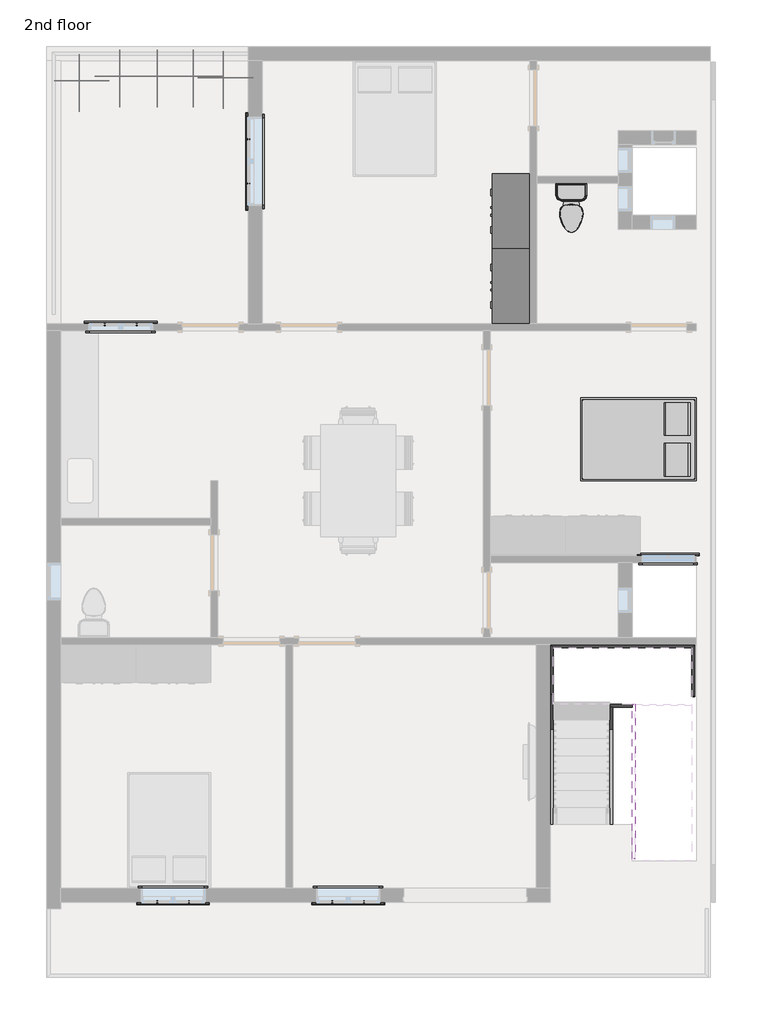
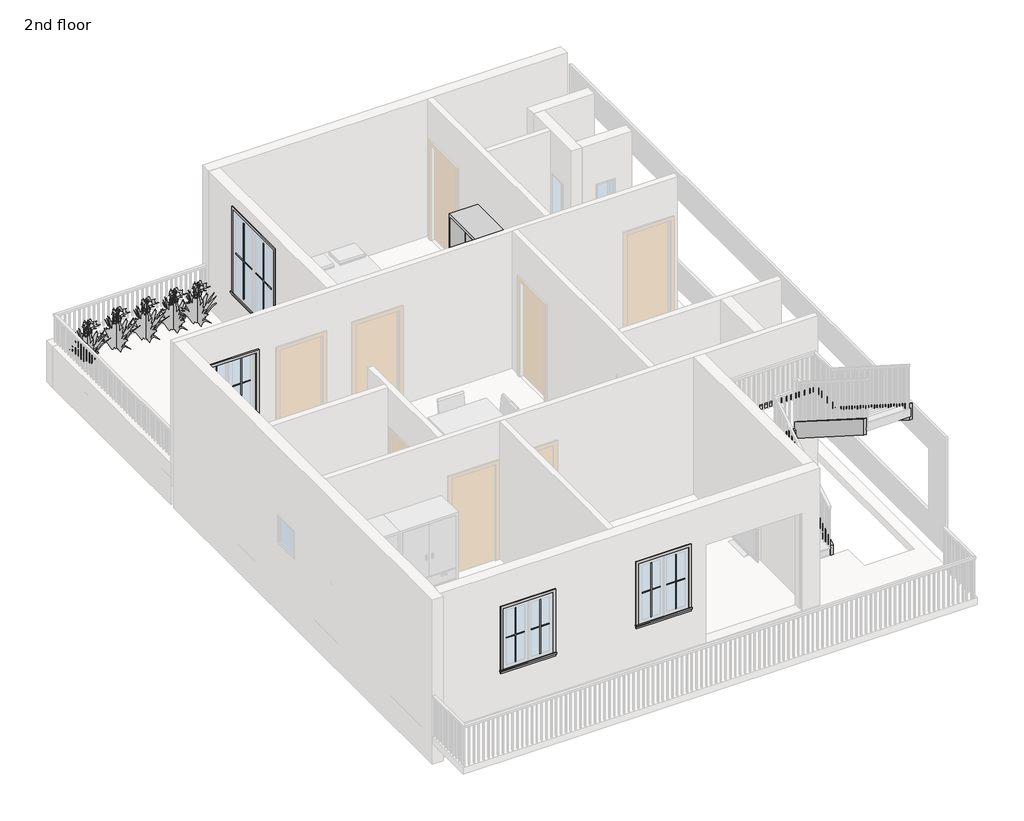
# One storey, part 5 of 5: 20 proxies, 8 members, 5 geographic elements, 3 furniture elements, 1 flow terminal.
"""IFC4 building model written with IfcOpenShell, lengths in millimetres."""

from ifc_helpers import new_model, si_unit, frame, origin, place, context, project, spatial, polyline, outline, extrude, faceted_brep, transform, mapped, element, save
from components import muntin_pattern_2x2_muntin_pattern_2x2_bff912c5, muntin_pattern_2x2_muntin_pattern_2x2_c2194282, muntin_pattern_2x2_muntin_pattern_2x2_88bf7f41, muntin_pattern_2x2_muntin_pattern_2x2_3dfd0a47, muntin_pattern_2x2_muntin_pattern_2x2_b3fe6957, muntin_pattern_2x2_muntin_pattern_2x2_3e0ecaf2, trim_window_exterior_flat_with_sill_e04b3088, trim_window_exterior_flat_with_sill_4930676f, trim_window_exterior_flat_with_sill_41619996, trim_window_interior_flat_picture_frame_2a7685fe, trim_window_interior_flat_picture_frame_dd064338, trim_window_interior_flat_picture_frame_51c85655, toilet_domestic_3d_toilet_domestic_3d_ba6479b0, toilet_domestic_3d_toilet_domestic_3d_30431060, furniture_b58f7881, furniture_82e269c4, rpc_plant_tropical_55f6ff97

model = new_model("IFC4")

# Units and contexts
model_context = context("Model", 3, world=origin())
ifc_project = project(units=[si_unit("LENGTHUNIT", "METRE", prefix="MILLI")], contexts=[model_context])

# Site, building, storey
site = spatial("IfcSite", under=ifc_project)
building = spatial("IfcBuilding", under=site)
storey = spatial("IfcBuildingStorey", under=building, Name="2nd floor", Elevation=7010.4)

# Proxies
placement = place(None, origin())
muntin_pattern_2x2_muntin_pattern_2x2_shape = muntin_pattern_2x2_muntin_pattern_2x2_bff912c5(model_context)
element("IfcBuildingElementProxy", 1, Name="Muntin Pattern_2x2 : Muntin Pattern_2x2", ObjectType="Muntin Pattern_2x2 : Muntin Pattern_2x2", at=placement, inside=storey, context=model_context, shape_type="MappedRepresentation", body=[
    mapped(muntin_pattern_2x2_muntin_pattern_2x2_shape, transform((-4824.2248597, 10579.5632925, 7994.65), x_axis=(0.0, 1.0, 0.0), y_axis=(-1.0, 0.0, 0.0), z_axis=(0.0, 0.0, 1.0))),
])
muntin_pattern_2x2_muntin_pattern_2x2_2_shape = muntin_pattern_2x2_muntin_pattern_2x2_c2194282(model_context)
element("IfcBuildingElementProxy", 2, Name="Muntin Pattern_2x2 : Muntin Pattern_2x2", ObjectType="Muntin Pattern_2x2 : Muntin Pattern_2x2", at=placement, inside=storey, context=model_context, shape_type="MappedRepresentation", body=[
    mapped(muntin_pattern_2x2_muntin_pattern_2x2_2_shape, transform((-4824.2248597, 11300.2882925, 7994.65), x_axis=(0.0, -1.0, 0.0), y_axis=(1.0, 0.0, 0.0), z_axis=(0.0, 0.0, 1.0))),
])
muntin_pattern_2x2_muntin_pattern_2x2_3_shape = muntin_pattern_2x2_muntin_pattern_2x2_88bf7f41(model_context)
element("IfcBuildingElementProxy", 3, Name="Muntin Pattern_2x2 : Muntin Pattern_2x2", ObjectType="Muntin Pattern_2x2 : Muntin Pattern_2x2", at=placement, inside=storey, context=model_context, shape_type="MappedRepresentation", body=[
    mapped(muntin_pattern_2x2_muntin_pattern_2x2_3_shape, transform((-7162.6123597, 8288.8007925, 7994.65), x_axis=(1.0, 0.0, 0.0), y_axis=(0.0, 1.0, 0.0), z_axis=(0.0, 0.0, 1.0))),
])
element("IfcBuildingElementProxy", 4, Name="Muntin Pattern_2x2 : Muntin Pattern_2x2", ObjectType="Muntin Pattern_2x2 : Muntin Pattern_2x2", at=placement, inside=storey, context=model_context, shape_type="MappedRepresentation", body=[
    mapped(muntin_pattern_2x2_muntin_pattern_2x2_3_shape, transform((-5794.1873597, -1102.8492075, 7994.65), x_axis=(-1.0, 0.0, 0.0), y_axis=(0.0, -1.0, 0.0), z_axis=(0.0, 0.0, 1.0))),
])
element("IfcBuildingElementProxy", 5, Name="Muntin Pattern_2x2 : Muntin Pattern_2x2", ObjectType="Muntin Pattern_2x2 : Muntin Pattern_2x2", at=placement, inside=storey, context=model_context, shape_type="MappedRepresentation", body=[
    mapped(muntin_pattern_2x2_muntin_pattern_2x2_3_shape, transform((-2946.0873597, -1102.8492075, 7994.65), x_axis=(-1.0, 0.0, 0.0), y_axis=(0.0, -1.0, 0.0), z_axis=(0.0, 0.0, 1.0))),
])
muntin_pattern_2x2_muntin_pattern_2x2_4_shape = muntin_pattern_2x2_muntin_pattern_2x2_3dfd0a47(model_context)
element("IfcBuildingElementProxy", 6, Name="Muntin Pattern_2x2 : Muntin Pattern_2x2", ObjectType="Muntin Pattern_2x2 : Muntin Pattern_2x2", at=placement, inside=storey, context=model_context, shape_type="MappedRepresentation", body=[
    mapped(muntin_pattern_2x2_muntin_pattern_2x2_4_shape, transform((-6645.0873597, 8288.8007925, 7994.65), x_axis=(-1.0, 0.0, 0.0), y_axis=(0.0, -1.0, 0.0), z_axis=(0.0, 0.0, 1.0))),
])
element("IfcBuildingElementProxy", 7, Name="Muntin Pattern_2x2 : Muntin Pattern_2x2", ObjectType="Muntin Pattern_2x2 : Muntin Pattern_2x2", at=placement, inside=storey, context=model_context, shape_type="MappedRepresentation", body=[
    mapped(muntin_pattern_2x2_muntin_pattern_2x2_4_shape, transform((-6311.7123597, -1102.8492075, 7994.65), x_axis=(1.0, 0.0, 0.0), y_axis=(0.0, 1.0, 0.0), z_axis=(0.0, 0.0, 1.0))),
])
element("IfcBuildingElementProxy", 8, Name="Muntin Pattern_2x2 : Muntin Pattern_2x2", ObjectType="Muntin Pattern_2x2 : Muntin Pattern_2x2", at=placement, inside=storey, context=model_context, shape_type="MappedRepresentation", body=[
    mapped(muntin_pattern_2x2_muntin_pattern_2x2_4_shape, transform((-3463.6123597, -1102.8492075, 7994.65), x_axis=(1.0, 0.0, 0.0), y_axis=(0.0, 1.0, 0.0), z_axis=(0.0, 0.0, 1.0))),
])
muntin_pattern_2x2_muntin_pattern_2x2_5_shape = muntin_pattern_2x2_muntin_pattern_2x2_b3fe6957(model_context)
element("IfcBuildingElementProxy", 9, Name="Muntin Pattern_2x2 : Muntin Pattern_2x2", ObjectType="Muntin Pattern_2x2 : Muntin Pattern_2x2", at=placement, inside=storey, context=model_context, shape_type="MappedRepresentation", body=[
    mapped(muntin_pattern_2x2_muntin_pattern_2x2_5_shape, transform((1784.5376403, 4516.9007925, 7385.05), x_axis=(1.0, 0.0, 0.0), y_axis=(0.0, 1.0, 0.0), z_axis=(0.0, 0.0, 1.0))),
])
muntin_pattern_2x2_muntin_pattern_2x2_6_shape = muntin_pattern_2x2_muntin_pattern_2x2_3e0ecaf2(model_context)
element("IfcBuildingElementProxy", 10, Name="Muntin Pattern_2x2 : Muntin Pattern_2x2", ObjectType="Muntin Pattern_2x2 : Muntin Pattern_2x2", at=placement, inside=storey, context=model_context, shape_type="MappedRepresentation", body=[
    mapped(muntin_pattern_2x2_muntin_pattern_2x2_6_shape, transform((2213.1626403, 4516.9007925, 7385.05), x_axis=(-1.0, 0.0, 0.0), y_axis=(0.0, -1.0, 0.0), z_axis=(0.0, 0.0, 1.0))),
])
trim_window_exterior_flat_with_sill_shape = trim_window_exterior_flat_with_sill_e04b3088(model_context)
element("IfcBuildingElementProxy", 11, Name="Trim-Window-Exterior-Flat : with Sill", ObjectType="Trim-Window-Exterior-Flat : with Sill", at=placement, inside=storey, context=model_context, shape_type="MappedRepresentation", body=[
    mapped(trim_window_exterior_flat_with_sill_shape, transform((-4833.7498597, 10939.9257925, 9753.6), x_axis=(0.0, -1.0, 0.0), y_axis=(0.0, 0.0, 1.0), z_axis=(-1.0, 0.0, 0.0))),
])
trim_window_exterior_flat_with_sill_2_shape = trim_window_exterior_flat_with_sill_4930676f(model_context)
element("IfcBuildingElementProxy", 12, Name="Trim-Window-Exterior-Flat : with Sill", ObjectType="Trim-Window-Exterior-Flat : with Sill", at=placement, inside=storey, context=model_context, shape_type="MappedRepresentation", body=[
    mapped(trim_window_exterior_flat_with_sill_2_shape, transform((-6903.8498597, 8298.3257925, 9271.0), x_axis=(-1.0, 0.0, 0.0), y_axis=(0.0, 0.0, 1.0), z_axis=(0.0, 1.0, 0.0))),
])
element("IfcBuildingElementProxy", 13, Name="Trim-Window-Exterior-Flat : with Sill", ObjectType="Trim-Window-Exterior-Flat : with Sill", at=placement, inside=storey, context=model_context, shape_type="MappedRepresentation", body=[
    mapped(trim_window_exterior_flat_with_sill_2_shape, transform((-6052.9498597, -1112.3742075, 9271.0), x_axis=(1.0, 0.0, 0.0), y_axis=(0.0, 0.0, 1.0), z_axis=(0.0, -1.0, 0.0))),
])
element("IfcBuildingElementProxy", 14, Name="Trim-Window-Exterior-Flat : with Sill", ObjectType="Trim-Window-Exterior-Flat : with Sill", at=placement, inside=storey, context=model_context, shape_type="MappedRepresentation", body=[
    mapped(trim_window_exterior_flat_with_sill_2_shape, transform((-3204.8498597, -1112.3742075, 9271.0), x_axis=(1.0, 0.0, 0.0), y_axis=(0.0, 0.0, 1.0), z_axis=(0.0, -1.0, 0.0))),
])
trim_window_exterior_flat_with_sill_3_shape = trim_window_exterior_flat_with_sill_41619996(model_context)
element("IfcBuildingElementProxy", 15, Name="Trim-Window-Exterior-Flat : with Sill", ObjectType="Trim-Window-Exterior-Flat : with Sill", at=placement, inside=storey, context=model_context, shape_type="MappedRepresentation", body=[
    mapped(trim_window_exterior_flat_with_sill_3_shape, transform((1998.8501403, 4526.4257925, 8229.6), x_axis=(-1.0, 0.0, 0.0), y_axis=(0.0, 0.0, 1.0), z_axis=(0.0, 1.0, 0.0))),
])
trim_window_interior_flat_picture_frame_shape = trim_window_interior_flat_picture_frame_2a7685fe(model_context)
element("IfcBuildingElementProxy", 16, Name="Trim-Window-Interior-Flat : Picture Frame", ObjectType="Trim-Window-Interior-Flat : Picture Frame", at=placement, inside=storey, context=model_context, shape_type="MappedRepresentation", body=[
    mapped(trim_window_interior_flat_picture_frame_shape, transform((-4605.1498597, 10939.9257925, 9753.6), x_axis=(0.0, 1.0, 0.0), y_axis=(0.0, 0.0, 1.0), z_axis=(1.0, 0.0, 0.0))),
])
trim_window_interior_flat_picture_frame_2_shape = trim_window_interior_flat_picture_frame_dd064338(model_context)
element("IfcBuildingElementProxy", 17, Name="Trim-Window-Interior-Flat : Picture Frame", ObjectType="Trim-Window-Interior-Flat : Picture Frame", at=placement, inside=storey, context=model_context, shape_type="MappedRepresentation", body=[
    mapped(trim_window_interior_flat_picture_frame_2_shape, transform((-6903.8498597, 8184.0257925, 9271.0), x_axis=(1.0, 0.0, 0.0), y_axis=(0.0, 0.0, 1.0), z_axis=(0.0, -1.0, 0.0))),
])
element("IfcBuildingElementProxy", 18, Name="Trim-Window-Interior-Flat : Picture Frame", ObjectType="Trim-Window-Interior-Flat : Picture Frame", at=placement, inside=storey, context=model_context, shape_type="MappedRepresentation", body=[
    mapped(trim_window_interior_flat_picture_frame_2_shape, transform((-6052.9498597, -883.7742075, 9271.0), x_axis=(-1.0, 0.0, 0.0), y_axis=(0.0, 0.0, 1.0), z_axis=(0.0, 1.0, 0.0))),
])
element("IfcBuildingElementProxy", 19, Name="Trim-Window-Interior-Flat : Picture Frame", ObjectType="Trim-Window-Interior-Flat : Picture Frame", at=placement, inside=storey, context=model_context, shape_type="MappedRepresentation", body=[
    mapped(trim_window_interior_flat_picture_frame_2_shape, transform((-3204.8498597, -883.7742075, 9271.0), x_axis=(-1.0, 0.0, 0.0), y_axis=(0.0, 0.0, 1.0), z_axis=(0.0, 1.0, 0.0))),
])
trim_window_interior_flat_picture_frame_3_shape = trim_window_interior_flat_picture_frame_51c85655(model_context)
element("IfcBuildingElementProxy", 20, Name="Trim-Window-Interior-Flat : Picture Frame", ObjectType="Trim-Window-Interior-Flat : Picture Frame", at=placement, inside=storey, context=model_context, shape_type="MappedRepresentation", body=[
    mapped(trim_window_interior_flat_picture_frame_3_shape, transform((1998.8501403, 4412.1257925, 8229.6), x_axis=(1.0, 0.0, 0.0), y_axis=(0.0, 0.0, 1.0), z_axis=(0.0, -1.0, 0.0))),
])

# Flow terminal
toilet_domestic_3d_toilet_domestic_3d_shape = toilet_domestic_3d_toilet_domestic_3d_ba6479b0(model_context)
toilet_domestic_3d_toilet_domestic_3d_2_shape = toilet_domestic_3d_toilet_domestic_3d_30431060(model_context)
element("IfcFlowTerminal", 21, ObjectType="Toilet-Domestic-3D : Toilet-Domestic-3D", at=placement, inside=storey, context=model_context, shape_type="MappedRepresentation", body=[
    mapped(toilet_domestic_3d_toilet_domestic_3d_shape, transform((424.0501403, 10089.0257925, 7010.4), x_axis=(1.0, 0.0, 0.0), y_axis=(0.0, 1.0, 0.0), z_axis=(0.0, 0.0, 1.0))),
    mapped(toilet_domestic_3d_toilet_domestic_3d_2_shape, transform((424.0501403, 10089.0257925, 7010.4), x_axis=(1.0, 0.0, 0.0), y_axis=(0.0, 1.0, 0.0), z_axis=(0.0, 0.0, 1.0))),
])

# Furniture
furniture_shape = furniture_b58f7881(model_context)
element("IfcFurniture", 22, ObjectType="Bed-Box : Double 53\" x 74\"", at=placement, inside=storey, context=model_context, shape_type="MappedRepresentation", body=[
    mapped(furniture_shape, transform((1750.6796485, 6757.8782516, 7010.4), x_axis=(0.0, -1.0, 0.0), y_axis=(1.0, 0.0, 0.0), z_axis=(0.0, 0.0, 1.0))),
])
furniture_2_shape = furniture_82e269c4(model_context)
element("IfcFurniture", 23, ObjectType="Wardrobe : 48\" x 72\" x 24\"", at=placement, inside=storey, context=model_context, shape_type="MappedRepresentation", body=[
    mapped(furniture_2_shape, transform((29.8889499, 8638.7325327, 7010.4), x_axis=(0.0, -1.0, 0.0), y_axis=(1.0, 0.0, 0.0), z_axis=(0.0, 0.0, 1.0))),
])
element("IfcFurniture", 24, ObjectType="Wardrobe : 48\" x 72\" x 24\"", at=placement, inside=storey, context=model_context, shape_type="MappedRepresentation", body=[
    mapped(furniture_2_shape, transform((29.8889499, 9857.9325327, 7010.4), x_axis=(0.0, -1.0, 0.0), y_axis=(1.0, 0.0, 0.0), z_axis=(0.0, 0.0, 1.0))),
])

# Geographic elements
rpc_plant_tropical_shape = rpc_plant_tropical_55f6ff97(model_context)
element("IfcGeographicElement", 25, ObjectType="RPC Plant - Tropical", at=placement, inside=storey, context=model_context, shape_type="MappedRepresentation", body=[
    mapped(rpc_plant_tropical_shape, transform((-7576.9498597, 12248.0257925, 7010.4), x_axis=(1.0, 0.0, 0.0), y_axis=(0.0, 1.0, 0.0), z_axis=(0.0, 0.0, 1.0))),
])
element("IfcGeographicElement", 26, ObjectType="RPC Plant - Tropical", at=placement, inside=storey, context=model_context, shape_type="MappedRepresentation", body=[
    mapped(rpc_plant_tropical_shape, transform((-5240.1498597, 12298.8257925, 7010.4), x_axis=(1.0, 0.0, 0.0), y_axis=(0.0, 1.0, 0.0), z_axis=(0.0, 0.0, 1.0))),
])
element("IfcGeographicElement", 27, ObjectType="RPC Plant - Tropical", at=placement, inside=storey, context=model_context, shape_type="MappedRepresentation", body=[
    mapped(rpc_plant_tropical_shape, transform((-6916.5498597, 12324.2257925, 7010.4), x_axis=(1.0, 0.0, 0.0), y_axis=(0.0, 1.0, 0.0), z_axis=(0.0, 0.0, 1.0))),
])
element("IfcGeographicElement", 28, ObjectType="RPC Plant - Tropical", at=placement, inside=storey, context=model_context, shape_type="MappedRepresentation", body=[
    mapped(rpc_plant_tropical_shape, transform((-6306.9498597, 12324.2257925, 7010.4), x_axis=(1.0, 0.0, 0.0), y_axis=(0.0, 1.0, 0.0), z_axis=(0.0, 0.0, 1.0))),
])
element("IfcGeographicElement", 29, ObjectType="RPC Plant - Tropical", at=placement, inside=storey, context=model_context, shape_type="MappedRepresentation", body=[
    mapped(rpc_plant_tropical_shape, transform((-5722.7498597, 12324.2257925, 7010.4), x_axis=(1.0, 0.0, 0.0), y_axis=(0.0, 1.0, 0.0), z_axis=(0.0, 0.0, 1.0))),
])

# Members
element("IfcMember", 30, ObjectType="Stringer - 2\" Width", at=placement, inside=storey, context=model_context, shape_type="SweptSolid", body=[
    extrude(outline(polyline([(157.6257925, 7010.4), (157.6257925, 7225.4106437), (2174.694781, 8509.0), (2263.4527505, 8204.2), (387.4813219, 7010.4), (157.6257925, 7010.4)])), frame((81.1501403, 0.0, 0.0), z_axis=(1.0, 0.0, 0.0), x_axis=(0.0, 1.0, 0.0)), (0.0, 0.0, 1.0), 50.8),
])
element("IfcMember", 31, ObjectType="Stringer - 2\" Width", at=placement, inside=storey, context=model_context, shape_type="SweptSolid", body=[
    extrude(outline(polyline([(157.6257925, 7010.4), (157.6257925, 7225.4106437), (2062.6257925, 8437.683371), (2062.6257925, 8076.4010268), (387.4813219, 7010.4), (157.6257925, 7010.4)])), frame((1046.3501403, 0.0, 0.0), z_axis=(1.0, 0.0, 0.0), x_axis=(0.0, 1.0, 0.0)), (0.0, 0.0, 1.0), 50.8),
])
element("IfcMember", 32, ObjectType="Stringer - 2\" Width", at=placement, inside=storey, context=model_context, shape_type="SweptSolid", body=[
    extrude(outline(polyline([(2331.5568041, 8509.0), (2242.7988346, 8204.2), (-401.1742075, 9886.7282995), (-401.1742075, 10248.0106437), (2331.5568041, 8509.0)])), frame((2379.8501403, 0.0, 0.0), z_axis=(1.0, 0.0, 0.0), x_axis=(0.0, 1.0, 0.0)), (0.0, 0.0, 1.0), 50.8),
])
element("IfcMember", 33, ObjectType="Stringer - 2\" Width", at=placement, inside=storey, context=model_context, shape_type="SweptSolid", body=[
    extrude(outline(polyline([(2113.4257925, 8647.8106437), (2113.4257925, 8286.5282995), (-401.1742075, 9886.7282995), (-401.1742075, 10248.0106437), (2113.4257925, 8647.8106437)])), frame((1414.6501403, 0.0, 0.0), z_axis=(1.0, 0.0, 0.0), x_axis=(0.0, 1.0, 0.0)), (0.0, 0.0, 1.0), 50.8),
])
element("IfcMember", 34, ObjectType="Stringer - 2\" Width", at=placement, inside=storey, context=model_context, shape_type="Brep", body=[
    faceted_brep([(2379.8501403, 2331.5568041, 8509.0), (2430.6501403, 2331.5568041, 8509.0), (2430.6501403, 3078.6257925, 8509.0), (2379.8501403, 3027.8257925, 8509.0), (2379.8501403, 2242.7988346, 8204.2), (2379.8501403, 3027.8257925, 8204.2), (2430.6501403, 2242.7988346, 8204.2), (2430.6501403, 3078.6257925, 8204.2)], [[[0, 1, 2, 3]], [[4, 0, 3, 5]], [[6, 4, 5, 7]], [[1, 6, 7, 2]], [[1, 0, 4, 6]], [[2, 7, 5, 3]]]),
])
element("IfcMember", 35, ObjectType="Stringer - 2\" Width", at=placement, inside=storey, context=model_context, shape_type="SweptSolid", body=[
    extrude(outline(polyline([(2430.6501403, 3078.6257925), (2379.8501403, 3027.8257925), (131.9501403, 3027.8257925), (81.1501403, 3078.6257925), (2430.6501403, 3078.6257925)])), frame((0.0, 0.0, 8204.2), z_axis=(0.0, 0.0, 1.0), x_axis=(1.0, 0.0, 0.0)), (0.0, 0.0, 1.0), 304.8),
])
element("IfcMember", 36, ObjectType="Stringer - 2\" Width", at=placement, inside=storey, context=model_context, shape_type="Brep", body=[
    faceted_brep([(131.9501403, 3027.8257925, 8509.0), (81.1501403, 3078.6257925, 8509.0), (81.1501403, 2174.694781, 8509.0), (131.9501403, 2174.694781, 8509.0), (131.9501403, 3027.8257925, 8204.2), (131.9501403, 2263.4527505, 8204.2), (81.1501403, 3078.6257925, 8204.2), (81.1501403, 2263.4527505, 8204.2)], [[[0, 1, 2, 3]], [[4, 0, 3, 5]], [[6, 4, 5, 7]], [[1, 6, 7, 2]], [[1, 0, 4, 6]], [[2, 7, 5, 3]]]),
])
element("IfcMember", 37, ObjectType="Stringer - 2\" Width", at=placement, inside=storey, context=model_context, shape_type="SweptSolid", body=[
    extrude(outline(polyline([(1046.3501403, 2062.6257925), (1046.3501403, 2113.4257925), (1414.6501403, 2113.4257925), (1414.6501403, 2062.6257925), (1046.3501403, 2062.6257925)])), frame((0.0, 0.0, 8204.2), z_axis=(0.0, 0.0, 1.0), x_axis=(1.0, 0.0, 0.0)), (0.0, 0.0, 1.0), 304.8),
])

save(model, "model.ifc")

# Revit data of these elements
# Type "Muntin Pattern_2x2 : Muntin Pattern_2x2"
#   Width [instance default] = 4' - 0"
#   Thickness = 0' - 0 1/2"
#   Height [instance default] = 4' - 0"
#   Distance = 0' - 0 3/4"
#   Interior Material [instance default] = none
#   Exterior Material [instance default] = none
#   Default Elevation = 0
# Type "Trim-Window-Exterior-Flat : with Sill"
#   Trim Width = 0' - 2 1/4"
#   Trim Thickness_Picture Frame = 0' - 1 1/4"
#   Trim Thickness_with Sill = 0' - 0 3/4"
#   Sill Thickness = 0' - 1 1/4"
#   Opening Width [instance default] = 2' - 0"
#   Opening Height [instance default] = 3' - 0"
#   Default Elevation = 4' - 0"
#   Sill = yes
#   Picture Frame = no
#   Trim Material [instance default] = none
# Type "Trim-Window-Interior-Flat : Picture Frame"
#   Trim Thickness_Picture Frame = 0' - 1 1/4"
#   Trim Width = 0' - 2 1/4"
#   Trim Thickness_with Sill = 0' - 0 3/4"
#   Sill Thickness = 0' - 1 1/4"
#   Opening Width [instance default] = 2' - 0"
#   Opening Height [instance default] = 3' - 0"
#   Default Elevation = 4' - 0"
#   Sill = no
#   Picture Frame = yes
#   Trim Material [instance default] = none
# Type "Toilet-Domestic-3D : Toilet-Domestic-3D"
#   Assembly Code = "D2010110"
#   Toilet - Bowl/Basin Material = Porcelain, Linen
#   Toilet - Seat Material = Laminate, Linen, Matte
#   Default Elevation = 0
# Type "Bed-Box : Double 53\" x 74\""
#   Assembly Code = "E2020200"
#   Length = 6' - 2"
#   Width = 4' - 5"
#   Frame Material = Birch
#   Mattress Material = Linen, White
#   Default Elevation = 0
# Type "Wardrobe : 48\" x 72\" x 24\""
#   Assembly Code = "E2020200"
#   Depth = 2' - 0"
#   Height = 6' - 0"
#   Width = 4' - 0"
#   Material = Wood - Mahogany
#   Default Elevation = 0
# Type "RPC Plant - Tropical"
#   built-in parameter 1005198 = "{2, 15},{39, RPC-16-FWM5-GM7X-C67P-4000-ST1L-LVER-AU},{1, 0},{1, 0},{2, 35},{1, 8},{5, Color},{1, 0},{1, 0},{3, 0.8},{3, 0.8},{3, 0.8},{1, 8},{7, BBoxMin},{1, 0},{1, 0},{1, 0},{1, 0},{1, 0},{1, 8},{7, BBoxMax},{1, 0},{1, 0},{1, 0},{1, 0},{1, 0},{2, 11},{9, RPCTypeId},{1, 0},{1, 0},{39, RPC-16-FWM5-GM7X-C67P-4000-ST1L-LVER-AU},{1, 6},{14, RPCPlantHeight},{1, 0},{1, 0},{1, 3},{2, 11},{7, keyword},{1, 0},{1, 0},{99, :Geometry:RPC:Crane Lily:strelitzia:reinae:crane lily:plants:shrub:flower:tropical:bird-of-paradise},{2, 11},{8, category},{1, 0},{1, 0},{17, :Shrubs [General]},{2, 11},{12, LocalizedUID},{1, 0},{1, 0},{10, Crane Lily},{2, 14},{6, Height},{1, 0},{1, 0},{1, 3},{1, 2},{16, Cast Reflections},{1, 0},{1, 0},{1, 0},{1, 2},{12, Cast Shadows},{1, 0},{1, 0},{1, 1},{1, 2},{9, Lock View},{1, 0},{1, 0},{1, 0},{1, 4},{5, ViewC},{1, 0},{1, 0},{1, 0},{2, 11},{20, AdvancedUIDefinition},{1, 0},{1, 0},{0, },{2, 11},{10, AssetLibID},{1, 0},{1, 0},{36, 4D3F6E72-3F99-4203-98E9-AF80B3C7A7A4},{2, 11},{10, BaseSchema},{1, 0},{1, 0},{9, RPCSchema},{2, 11},{12, ExchangeGUID},{1, 0},{1, 0},{0, },{1, 2},{6, Hidden},{1, 0},{1, 0},{1, 0},{1, 4},{11, RPCCategory},{1, 0},{1, 0},{1, 0},{2, 11},{8, RPCImage},{1, 0},{1, 0},{0, },{1, 4},{13, SchemaVersion},{1, 0},{1, 0},{1, 4},{2, 11},{12, UIDefinition},{1, 0},{1, 0},{0, },{2, 11},{6, UIName},{1, 0},{1, 0},{39, RPC-16-FWM5-GM7X-C67P-4000-ST1L-LVER-AU},{2, 11},{11, VersionGUID},{1, 0},{1, 0},{9, RPCSchema},{2, 11},{9, assettype},{1, 0},{1, 0},{11, RPCGeometry},{2, 11},{11, description},{1, 0},{1, 0},{0, },{2, 11},{9, localname},{1, 0},{1, 0},{3, RPC},{2, 11},{9, localtype},{1, 0},{1, 0},{3, RPC},{1, 4},{8, revision},{1, 0},{1, 0},{1, 1},{2, 11},{9, thumbnail},{1, 0},{1, 0},{0, },{1, 4},{7, version},{1, 0},{1, 0},{1, 1},{1, 2},{20, RPC_Cast Reflections},{1, 0},{1, 0},{1, 1},{1, 2},{16, RPC_Cast Shadows},{1, 0},{1, 0},{1, 1},{1, 2},{13, RPC_Lock View},{1, 0},{1, 0},{1, 0},{1, 4},{9, RPC_ViewC},{1, 0},{1, 0},{1, 0},{21, assetlibrary_base.fbx},{1, 5},"
#   built-in parameter 1005195 = "RPC-16-FWM5-GM7X-C67P-4000-ST1L-LVER-AU"
#   Assembly Code = "G2050500"
#   Height = 3' - 0"
#   Default Elevation = 0
# Elements 1, 2 (IfcBuildingElementProxy, "Muntin Pattern_2x2 : Muntin Pattern_2x2")
#   Width = 1' - 11 1/8"
#   Height = 5' - 6 1/2"
#   Interior Material = Wood - Stained
#   Exterior Material = Clad - White
#   Phase Created = New Construction
#   Materials on its faces: "Clad - White", "Wood - Stained"
# Elements 3, 4, 5, 6, 7, 8 (IfcBuildingElementProxy, "Muntin Pattern_2x2 : Muntin Pattern_2x2")
#   Width = 1' - 3 1/8"
#   Height = 3' - 11 1/2"
#   Interior Material = Wood - Stained
#   Exterior Material = Clad - White
#   Phase Created = New Construction
#   Materials on its faces: "Clad - White", "Wood - Stained"
# Elements 9, 10 (IfcBuildingElementProxy, "Muntin Pattern_2x2 : Muntin Pattern_2x2")
#   Width = 0' - 11 5/8"
#   Height = 2' - 6 1/2"
#   Interior Material = Wood - Stained
#   Exterior Material = Clad - White
#   Phase Created = New Construction
#   Materials on its faces: "Clad - White", "Wood - Stained"
# Element 11 (IfcBuildingElementProxy, "Trim-Window-Exterior-Flat : with Sill")
#   Opening Width = 4' - 9"
#   Opening Height = 6' - 0"
#   Trim Material = Clad - White
#   Phase Created = New Construction
#   Materials on its faces: "Clad - White"
# Elements 12, 13, 14 (IfcBuildingElementProxy, "Trim-Window-Exterior-Flat : with Sill")
#   Opening Width = 3' - 5"
#   Opening Height = 4' - 5"
#   Trim Material = Clad - White
#   Phase Created = New Construction
#   Materials on its faces: "Clad - White"
# Element 15 (IfcBuildingElementProxy, "Trim-Window-Exterior-Flat : with Sill")
#   Opening Width = 2' - 10"
#   Opening Height = 3' - 0"
#   Trim Material = Clad - White
#   Phase Created = New Construction
#   Materials on its faces: "Clad - White"
# Element 16 (IfcBuildingElementProxy, "Trim-Window-Interior-Flat : Picture Frame")
#   Opening Width = 4' - 9"
#   Opening Height = 6' - 0"
#   Trim Material = Wood - Stained
#   Phase Created = New Construction
#   Materials on its faces: "Wood - Stained"
# Elements 17, 18, 19 (IfcBuildingElementProxy, "Trim-Window-Interior-Flat : Picture Frame")
#   Opening Width = 3' - 5"
#   Opening Height = 4' - 5"
#   Trim Material = Wood - Stained
#   Phase Created = New Construction
#   Materials on its faces: "Wood - Stained"
# Element 20 (IfcBuildingElementProxy, "Trim-Window-Interior-Flat : Picture Frame")
#   Opening Width = 2' - 10"
#   Opening Height = 3' - 0"
#   Trim Material = Wood - Stained
#   Phase Created = New Construction
#   Materials on its faces: "Wood - Stained"
# Element 21 (IfcFlowTerminal, "Toilet-Domestic-3D : Toilet-Domestic-3D")
#   Mark = "10"
#   Phase Created = New Construction
#   Materials on its faces: "Porcelain, Linen", "Laminate, Linen, Matte"
# Element 22 (IfcFurniture, "Bed-Box : Double 53\" x 74\"")
#   Phase Created = New Construction
#   Materials on its faces: "Birch", "Linen, White"
# Elements 23, 24 (IfcFurniture, "Wardrobe : 48\" x 72\" x 24\"")
#   Phase Created = New Construction
#   Materials on its faces: "Wood - Mahogany"
# Elements 25, 26, 27, 28, 29 (IfcGeographicElement, "RPC Plant - Tropical")
#   Phase Created = New Construction
# Elements 30, 31, 32, 33, 34, 35, 36, 37 (IfcMember, "Stringer - 2\" Width")
#   Phase Created = New Construction
# Materials
#   "Porcelain, Linen": class "Ceramic", colour RGB 249 239 230, transparency 0, Description = "Porcelain, linen", Cost = 0
#   "Laminate, Linen, Matte": class "Plastic", colour RGB 249 239 230, transparency 0, Description = "Plastic Laminate - Linen, Matte", Cost = 0
#   "Birch": class "Wood", colour RGB 224 178 126, transparency 0, Description = "Betula Alleghaniensis", Cost = 0
#   "Linen, White": class "Textile", colour RGB 247 247 239, transparency 0, Description = "Linen, white", Cost = 0
#   "Wood - Mahogany": colour RGB 138 86 45, transparency 0
#   "Clad - White": class "Wood", colour RGB 242 242 238, transparency 0, Cost = 0
#   "Wood - Stained": class "Wood", colour RGB 224 178 126, transparency 0, Cost = 0
